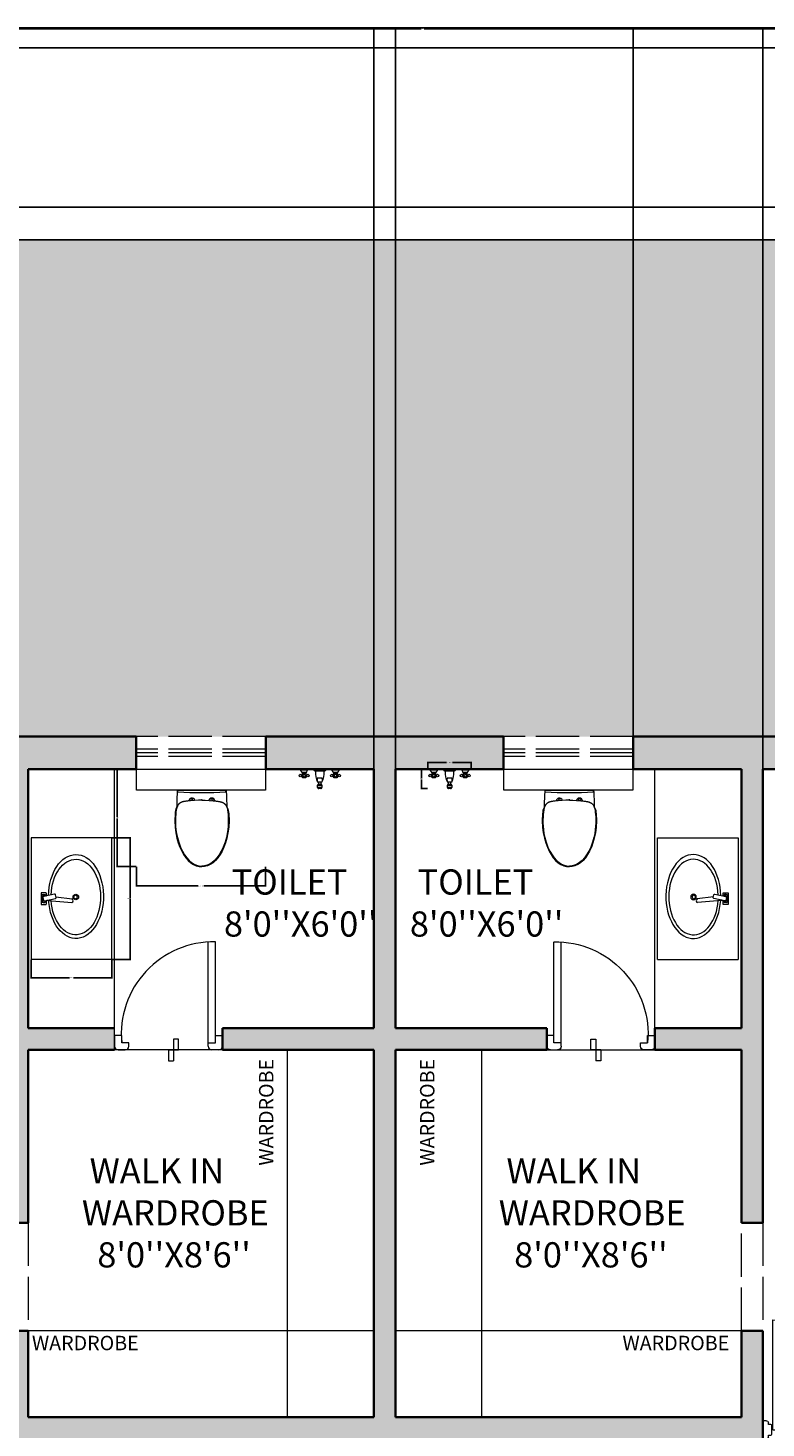
# Model space of a CAD drawing. Units: inches. Extents: x 84 to 1044, y -280 to 906.
# Tile 65 of 105: x 440 to 645, y 517 to 906. Entities that reach past the tile are written whole.
import ezdxf

# ---------------------------------------------------------------- set-up
doc = ezdxf.new("R2010")
doc.units = ezdxf.units.IN
doc.linetypes.add('ACAD_ISO02W100', pattern=[15, 12, -3])
for name, color, linetype, lineweight in [('00 FURNITURE', 15, 'Continuous', 15), ('A-ANNO-DIMS', 2, 'Continuous', 18), ('A-ANNO-TEXT', 7, 'Continuous', 13), ('A-ANNO-TTLB', 7, 'Continuous', 25), ('A-AREA-IDEN', 7, 'Continuous', 13), ('A-DOOR', 4, 'Continuous', 18), ('A-FLOR-CASE', 8, 'Continuous', 18), ('A-FLOR-FIXT', 9, 'Continuous', 15), ('A-GLAZ-HIGH', 160, 'ACAD_ISO02W100', 13), ('A-WALL-OVHD', 8, 'ACAD_ISO02W100', 13), ('A_FUR 1', 5, 'Continuous', 5), ('C-PROP', 7, 'Continuous', 25), ('WALL', 250, 'Continuous', 35)]:
    doc.layers.add(name, color=color, linetype=linetype, lineweight=lineweight)
doc.layers.add('A-WALL-PATT', color=251, linetype='Continuous', lineweight=9, true_color=0x636466)
doc.layers.add('L-PLNT-PATT', color=9, linetype='Continuous', lineweight=9, true_color=0xafd9aa)
doc.styles.add('1-100DIM', font='txt', dxfattribs={"height": 0.3})
doc.styles.get("Standard").update_dxf_attribs({"font": 'arial.ttf'})
doc.dimstyles.get("Standard").update_dxf_attribs({"dimtxt": 0.18, "dimasz": 0.18, "dimexe": 0.18, "dimexo": 0.0625, "dimgap": 0.09, "dimtad": 0, "dimtih": 1, "dimtoh": 1, "dimdec": 4, "dimzin": 0, "dimdsep": 46, "dimtxsty": 'Standard', "dimcen": 0.09, "dimadec": 0, "dimazin": 0, "dimtfac": 1, "dimtdec": 4, "dimtofl": 0, "dimtmove": 0, "dimatfit": 3, "dimfxl": 1, "dimtolj": 1, "dimtzin": 0, "dimarcsym": 0})

# ---------------------------------------------------------------- blocks, each defined once
blk = doc.blocks.new('DDD')
at = {"layer": '00 FURNITURE'}
for p, q in [((-12579.77, -15859.53), (-12579.77, -15829.05)), ((-12578.77, -15859.53), (-12578.77, -15829.03)), ((-12612.02, -15857.03), (-12612.02, -15862.03)), ((-12611.02, -15857.03), (-12612.02, -15857.03)), ((-12610.52, -15858.03), (-12610.52, -15857.53)), ((-12577.52, -15858.03), (-12577.52, -15857.53)), ((-12577.02, -15857.03), (-12576.02, -15857.03)), ((-12576.02, -15857.03), (-12576.02, -15862.03)), ((-12612.02, -15862.03), (-12611.02, -15862.03)), ((-12610.52, -15861.53), (-12610.52, -15861.03)), ((-12578.77, -15859.53), (-12579.77, -15859.53)), ((-12577.52, -15861.53), (-12577.52, -15861.03)), ((-12576.02, -15862.03), (-12577.02, -15862.03))]:
    blk.add_line(p, q, dxfattribs=at)
for points in [[(-12610.52, -15861.03), (-12610.02, -15861.03, 0.414214), (-12609.52, -15860.53), (-12609.52, -15858.53, 0.414214), (-12610.02, -15858.03), (-12610.52, -15858.03)], [(-12577.52, -15861.03), (-12578.02, -15861.03, -0.414214), (-12578.52, -15860.53), (-12578.52, -15858.53, -0.414214), (-12578.02, -15858.03), (-12577.52, -15858.03)]]:
    blk.add_lwpolyline(points, format="xyb", dxfattribs=at)
for centre, radius, start, end in [((-12578.77, -15859.53), 30.5, 90, 180), ((-12611.02, -15857.53), 0.5, 0, 90), ((-12577.02, -15857.53), 0.5, 90, 180), ((-12611.02, -15861.53), 0.5, 270, 0), ((-12577.02, -15861.53), 0.5, 180, 270)]:
    blk.add_arc(centre, radius, start, end, dxfattribs=at)
blk = doc.blocks.new('ESTSET')
at = {"layer": 'A_FUR 1'}
for p, q in [((-10.44, 4.1), (-10.44, 32.1)), ((-8.44, 4.1), (-8.44, 32.1)), ((-36.44, 6.1), (-36.44, 3.1)), ((-34.44, 6.1), (-36.44, 6.1)), ((-34.44, 4.1), (-34.44, 6.1)), ((-34.44, 4.1), (-34.44, 6.1)), ((-32.44, 4.1), (-34.44, 4.1)), ((-32.44, 4.1), (-34.44, 4.1)), ((-32.44, 3.1), (-32.44, 4.1)), ((-10.44, 3.1), (-10.44, 4.1)), ((-10.44, 4.1), (-8.44, 4.1)), ((-10.44, 4.1), (-8.44, 4.1)), ((-8.44, 4.1), (-8.44, 6.1)), ((-8.44, 6.1), (-6.44, 6.1)), ((-8.44, 4.1), (-8.44, 6.1)), ((-6.44, 6.1), (-6.44, 3.1)), ((-6.44, 2.1), (-36.44, 2.1)), ((-35.44, 2.1), (-33.44, 2.1)), ((-7.44, 2.1), (-9.44, 2.1))]:
    blk.add_line(p, q, dxfattribs=at)
for points in [[(-21.44, 2.1), (-18.67, 2.1), (-18.67, 5.1), (-20.06, 5.1)], [(-20.06, 5.1), (-20.06, -0.91)], [(-21.44, 2.1), (-21.44, -0.91), (-20.06, -0.91)]]:
    blk.add_lwpolyline(points, dxfattribs=at)
for centre, radius, start, end in [((-8.91, 6.46), 25.64, 88.9606, 185.2816), ((-35.44, 3.1), 1, 180, 270), ((-33.44, 3.1), 1, 270, 0), ((-9.44, 3.1), 1, 180, 270), ((-7.44, 3.1), 1, 270, 0)]:
    blk.add_arc(centre, radius, start, end, dxfattribs=at)
blk = doc.blocks.new('32')
at = {"layer": '00 FURNITURE'}
for p, q in [((-6.82, 0), (6.82, 0)), ((-6.68, -0.51), (-6.68, 0)), ((6.24, 0), (6.68, 0)), ((6.68, -0.51), (6.68, 0)), ((-6.41, -3.88), (-6.45, -3.92)), ((-6.38, -3.85), (-6.41, -3.88)), ((-6.34, -3.81), (-6.38, -3.85)), ((-6.31, -3.78), (-6.34, -3.81)), ((-6.27, -3.75), (-6.31, -3.78)), ((-6.24, -3.72), (-6.27, -3.75)), ((-6.2, -3.69), (-6.24, -3.72)), ((-6.16, -3.66), (-6.2, -3.69)), ((-6.13, -3.63), (-6.16, -3.66)), ((-6.09, -3.61), (-6.13, -3.63)), ((-6.05, -3.58), (-6.09, -3.61)), ((-6.01, -3.56), (-6.05, -3.58)), ((-5.98, -3.53), (-6.01, -3.56)), ((-5.94, -3.51), (-5.98, -3.53)), ((-5.91, -3.49), (-5.94, -3.51)), ((-5.87, -3.47), (-5.91, -3.49)), ((-5.83, -3.46), (-5.87, -3.47)), ((-5.8, -3.44), (-5.83, -3.46)), ((-5.76, -3.42), (-5.8, -3.44)), ((-5.73, -3.41), (-5.76, -3.42)), ((-5.7, -3.39), (-5.73, -3.41)), ((-5.66, -3.38), (-5.7, -3.39)), ((-5.63, -3.36), (-5.66, -3.38)), ((-5.6, -3.35), (-5.63, -3.36)), ((-5.57, -3.34), (-5.6, -3.35)), ((-5.53, -3.33), (-5.57, -3.34)), ((-5.5, -3.32), (-5.53, -3.33)), ((-5.47, -3.31), (-5.5, -3.32)), ((-5.44, -3.3), (-5.47, -3.31)), ((-5.41, -3.29), (-5.44, -3.3)), ((-5.39, -3.28), (-5.41, -3.29)), ((-5.36, -3.27), (-5.39, -3.28)), ((-5.33, -3.26), (-5.36, -3.27)), ((-5.3, -3.26), (-5.33, -3.26)), ((-5.27, -3.25), (-5.3, -3.26)), ((-5.25, -3.24), (-5.27, -3.25)), ((-5.22, -3.24), (-5.25, -3.24)), ((-5.19, -3.23), (-5.22, -3.24)), ((-5.17, -3.22), (-5.19, -3.23)), ((-5.15, -3.22), (-5.17, -3.22)), ((-5.12, -3.21), (-5.15, -3.22)), ((-5.1, -3.21), (-5.12, -3.21)), ((-5.08, -3.2), (-5.1, -3.21)), ((-5.05, -3.2), (-5.08, -3.2)), ((-5.03, -3.2), (-5.05, -3.2)), ((-5.01, -3.19), (-5.03, -3.2)), ((-4.97, -3.19), (-5.01, -3.19)), ((-4.93, -3.18), (-4.97, -3.19)), ((-4.89, -3.17), (-4.93, -3.18)), ((-4.86, -3.17), (-4.89, -3.17)), ((-4.82, -3.16), (-4.86, -3.17)), ((-4.78, -3.15), (-4.82, -3.16)), ((-4.72, -3.15), (-4.78, -3.15)), ((-4.63, -3.13), (-4.72, -3.15)), ((-4.46, -3.11), (-4.64, -3.14)), ((-4.34, -3.09), (-4.46, -3.11)), ((-4.15, -3.07), (-4.34, -3.09)), ((-3.99, -3.05), (-4.15, -3.07)), ((-3.77, -3.02), (-3.99, -3.05)), ((-3.5, -2.99), (-3.77, -3.02)), ((-3.34, -2.97), (-3.5, -2.99)), ((-3.3, -2.97), (-3.32, -2.97)), ((-3.26, -2.96), (-3.3, -2.97)), ((-3.21, -2.96), (-3.26, -2.96)), ((-3.15, -2.95), (-3.2, -2.96)), ((-2.01, -2.84), (-3.15, -2.95)), ((-0.94, -2.78), (-2.01, -2.84)), ((0, -2.76), (-0.94, -2.78)), ((0.12, -2.71), (-0.12, -2.71)), ((0, -2.76), (0.94, -2.78)), ((0.94, -2.78), (2.01, -2.84)), ((2.01, -2.84), (3.15, -2.95)), ((3.15, -2.95), (3.2, -2.96)), ((3.21, -2.96), (3.26, -2.96)), ((3.26, -2.96), (3.3, -2.97)), ((3.3, -2.97), (3.32, -2.97)), ((3.34, -2.97), (3.5, -2.99)), ((3.5, -2.99), (3.77, -3.02)), ((3.77, -3.02), (3.99, -3.05)), ((3.99, -3.05), (4.15, -3.07)), ((4.15, -3.07), (4.34, -3.09)), ((4.34, -3.09), (4.46, -3.11)), ((4.46, -3.11), (4.64, -3.14)), ((4.63, -3.13), (4.72, -3.15)), ((4.72, -3.15), (4.78, -3.15)), ((4.78, -3.15), (4.82, -3.16)), ((4.82, -3.16), (4.86, -3.17)), ((4.86, -3.17), (4.89, -3.17)), ((4.89, -3.17), (4.93, -3.18)), ((4.93, -3.18), (4.97, -3.19)), ((4.97, -3.19), (5.01, -3.19)), ((5.01, -3.19), (5.03, -3.2)), ((5.03, -3.2), (5.05, -3.2)), ((5.05, -3.2), (5.08, -3.2)), ((5.08, -3.2), (5.1, -3.21)), ((5.1, -3.21), (5.12, -3.21)), ((5.12, -3.21), (5.15, -3.22)), ((5.15, -3.22), (5.17, -3.22)), ((5.17, -3.22), (5.19, -3.23)), ((5.19, -3.23), (5.22, -3.24)), ((5.22, -3.24), (5.25, -3.24)), ((5.25, -3.24), (5.27, -3.25)), ((5.27, -3.25), (5.3, -3.26)), ((5.3, -3.26), (5.33, -3.26)), ((5.33, -3.26), (5.36, -3.27)), ((5.36, -3.27), (5.39, -3.28)), ((5.39, -3.28), (5.41, -3.29)), ((5.41, -3.29), (5.44, -3.3)), ((5.44, -3.3), (5.47, -3.31)), ((5.47, -3.31), (5.5, -3.32)), ((5.5, -3.32), (5.53, -3.33)), ((5.53, -3.33), (5.57, -3.34)), ((5.57, -3.34), (5.6, -3.35)), ((5.6, -3.35), (5.63, -3.36)), ((5.63, -3.36), (5.66, -3.38)), ((5.66, -3.38), (5.7, -3.39)), ((5.7, -3.39), (5.73, -3.41)), ((5.73, -3.41), (5.76, -3.42)), ((5.76, -3.42), (5.8, -3.44)), ((5.8, -3.44), (5.83, -3.46)), ((5.83, -3.46), (5.87, -3.47)), ((5.87, -3.47), (5.91, -3.49)), ((5.91, -3.49), (5.94, -3.51)), ((5.94, -3.51), (5.98, -3.53)), ((5.98, -3.53), (6.01, -3.56)), ((6.01, -3.56), (6.05, -3.58)), ((6.05, -3.58), (6.09, -3.61)), ((6.09, -3.61), (6.13, -3.63)), ((6.13, -3.63), (6.16, -3.66)), ((6.16, -3.66), (6.2, -3.69)), ((6.2, -3.69), (6.24, -3.72)), ((6.24, -3.72), (6.27, -3.75)), ((6.27, -3.75), (6.31, -3.78)), ((6.31, -3.78), (6.34, -3.81)), ((6.34, -3.81), (6.38, -3.85)), ((6.38, -3.85), (6.41, -3.88)), ((6.41, -3.88), (6.45, -3.92)), ((-7.44, -6.63), (-7.53, -8.53)), ((-7.39, -6.15), (-7.44, -6.62)), ((-7.32, -5.67), (-7.39, -6.15)), ((-7.31, -7.51), (-7.34, -8.28)), ((-7.21, -5.24), (-7.32, -5.67)), ((-7.27, -6.79), (-7.31, -7.51)), ((-7.21, -6.12), (-7.27, -6.79)), ((-7.01, -4.86), (-7.21, -5.24)), ((-7.13, -5.49), (-7.21, -6.12)), ((-6.99, -4.9), (-7.13, -5.49)), ((-6.93, -4.76), (-7.01, -4.86)), ((-6.79, -4.42), (-6.99, -4.9)), ((-6.77, -4.39), (-6.79, -4.42)), ((-6.74, -4.33), (-6.77, -4.39)), ((-6.71, -4.28), (-6.74, -4.33)), ((-6.67, -4.22), (-6.71, -4.28)), ((-6.64, -4.17), (-6.67, -4.22)), ((-6.61, -4.13), (-6.64, -4.17)), ((-6.58, -4.08), (-6.61, -4.13)), ((-6.55, -4.04), (-6.58, -4.08)), ((-6.51, -4), (-6.55, -4.04)), ((-6.48, -3.96), (-6.51, -4)), ((-6.45, -3.92), (-6.48, -3.96)), ((6.45, -3.92), (6.48, -3.96)), ((6.48, -3.96), (6.51, -4)), ((6.51, -4), (6.55, -4.04)), ((6.55, -4.04), (6.58, -4.08)), ((6.58, -4.08), (6.61, -4.13)), ((6.61, -4.13), (6.64, -4.17)), ((6.64, -4.17), (6.67, -4.22)), ((6.67, -4.22), (6.71, -4.28)), ((6.71, -4.28), (6.74, -4.33)), ((6.74, -4.33), (6.77, -4.39)), ((6.77, -4.39), (6.79, -4.42)), ((6.79, -4.42), (6.99, -4.9)), ((6.93, -4.76), (7.01, -4.86)), ((6.99, -4.9), (7.13, -5.49)), ((7.01, -4.86), (7.21, -5.24)), ((7.13, -5.49), (7.21, -6.12)), ((7.21, -5.24), (7.32, -5.67)), ((7.21, -6.12), (7.27, -6.79)), ((7.27, -6.79), (7.31, -7.51)), ((7.31, -7.51), (7.34, -8.28)), ((7.32, -5.67), (7.39, -6.15)), ((7.39, -6.15), (7.44, -6.62)), ((7.44, -6.63), (7.53, -8.53)), ((-7.53, -8.53), (-7.45, -10.3)), ((-7.45, -10.3), (-7.24, -11.89)), ((-7.34, -8.28), (-7.34, -9.11)), ((-7.34, -9.11), (-7.3, -10)), ((-7.3, -10), (-7.21, -10.97)), ((-7.21, -10.97), (-7.06, -12.03)), ((7.21, -10.97), (7.06, -12.03)), ((7.3, -10), (7.21, -10.97)), ((7.45, -10.3), (7.24, -11.89)), ((7.34, -9.11), (7.3, -10)), ((7.34, -8.28), (7.34, -9.11)), ((7.53, -8.53), (7.45, -10.3)), ((-7.24, -11.89), (-6.93, -13.34)), ((-7.06, -12.03), (-6.81, -13.19)), ((-6.93, -13.34), (-6.55, -14.65)), ((-6.81, -13.19), (-6.44, -14.48)), ((-6.55, -14.65), (-6.11, -15.85)), ((-6.44, -14.48), (-5.95, -15.8)), ((6.44, -14.48), (5.95, -15.8)), ((6.55, -14.65), (6.11, -15.85)), ((6.81, -13.19), (6.44, -14.48)), ((6.93, -13.34), (6.55, -14.65)), ((7.06, -12.03), (6.81, -13.19)), ((7.24, -11.89), (6.93, -13.34)), ((-6.11, -15.85), (-5.61, -16.94)), ((-5.95, -15.8), (-5.38, -16.99)), ((-5.61, -16.94), (-5.06, -17.92)), ((-5.38, -16.99), (-4.79, -17.98)), ((-5.06, -17.92), (-4.45, -18.78)), ((-4.79, -17.98), (-4.17, -18.83)), ((-4.45, -18.78), (-3.8, -19.54)), ((-4.17, -18.83), (-3.53, -19.54)), ((4.17, -18.83), (3.53, -19.54)), ((4.45, -18.78), (3.8, -19.54)), ((4.79, -17.98), (4.17, -18.83)), ((5.06, -17.92), (4.45, -18.78)), ((5.38, -16.99), (4.79, -17.98)), ((5.61, -16.94), (5.06, -17.92)), ((5.95, -15.8), (5.38, -16.99)), ((6.11, -15.85), (5.61, -16.94)), ((-3.8, -19.54), (-3.09, -20.17)), ((-3.53, -19.54), (-2.86, -20.12)), ((-3.09, -20.17), (-2.34, -20.67)), ((-2.86, -20.12), (-2.18, -20.55)), ((-2.34, -20.67), (-1.55, -21.01)), ((-2.18, -20.55), (-1.47, -20.85)), ((-1.55, -21.01), (-0.75, -21.2)), ((-1.47, -20.85), (-0.74, -21.03)), ((-0.75, -21.2), (0, -21.25)), ((-0.74, -21.03), (0, -21.08)), ((0.74, -21.03), (0, -21.08)), ((0.75, -21.2), (0, -21.25)), ((1.47, -20.85), (0.74, -21.03)), ((1.55, -21.01), (0.75, -21.2)), ((2.18, -20.55), (1.47, -20.85)), ((2.34, -20.67), (1.55, -21.01)), ((2.86, -20.12), (2.18, -20.55)), ((3.09, -20.17), (2.34, -20.67)), ((3.53, -19.54), (2.86, -20.12)), ((3.8, -19.54), (3.09, -20.17))]:
    blk.add_line(p, q, dxfattribs=at)
for points in [[(-6.82, 0), (-6.91, -1.63), (-6.97, -3.26), (-7.01, -4.89)], [(7.01, -4.89), (6.97, -3.26), (6.91, -1.63), (6.82, 0)], [(-6.68, -0.51), (-2.23, -0.73), (2.23, -0.73), (6.68, -0.51)], [(-2.97, -2.23), (-3.33, -2.32), (-3.59, -2.63), (-3.61, -3)], [(-1.94, -2.84), (-2.06, -2.38), (-2.52, -2.11), (-2.97, -2.23)], [(-2.58, -2.49), (-2.63, -2.45), (-2.7, -2.43), (-2.76, -2.43)], [(-2.54, -2.89), (-2.44, -2.77), (-2.46, -2.59), (-2.58, -2.49)], [(2.76, -2.2), (2.38, -2.2), (2.04, -2.46), (1.94, -2.84)], [(3.61, -3), (3.58, -2.55), (3.21, -2.2), (2.76, -2.2)], [(2.98, -2.53), (2.93, -2.46), (2.85, -2.43), (2.76, -2.43)], [(2.95, -2.93), (3.07, -2.83), (3.08, -2.65), (2.98, -2.53)]]:
    blk.add_open_spline(points, degree=3, dxfattribs=at)
for points in [[(-2.76, -2.43), (-2.92, -2.43), (-3.05, -2.56), (-3.05, -2.71), (-3.05, -2.8), (-3.01, -2.88), (-2.95, -2.93)], [(2.76, -2.43), (2.6, -2.43), (2.48, -2.56), (2.48, -2.71), (2.48, -2.78), (2.5, -2.84), (2.54, -2.89)]]:
    blk.add_open_spline(points, degree=3, knots=[0, 0, 0, 0, 1, 1, 1, 2, 2, 2, 2], dxfattribs=at)
blk = doc.blocks.new('WWCC')
at = {"layer": '00 FURNITURE', "ltscale": 20}
blk.add_lwpolyline([(140241.58, -48678.24), (140247.43, -48678.24), (140247.43, -48714.06), (140241.58, -48714.06)], close=True, dxfattribs=at)
at = {"layer": '00 FURNITURE', "rotation": 90.00000000000003}
blk.add_blockref('32', (140247.43, -48695.89), dxfattribs=at)
blk = doc.blocks.new('Faucet - Bathroom front')
for p, q in [((-0.5, 4.25), (0.5, 4.25)), ((0.5, 3.75), (-0.5, 3.75)), ((-0.25, 3), (-0.25, 3.5)), ((0.25, 3.5), (0.25, 3)), ((-5, 0), (-2.25, 0)), ((-4.5087, 0.25), (-2.7408, 0.25)), ((-4, 1.625), (-4.25, 1.625)), ((-4, 1.375), (-4.25, 1.375)), ((-3.1442, 0.75), (-4.0979, 0.75)), ((-3.25, 1.625), (-3, 1.625)), ((-3.25, 1.375), (-3, 1.375)), ((-1.5, 0), (1.5, 0)), ((-1, 0.5), (1, 0.5)), ((-0.5, 3), (0.5, 3)), ((0.5, 2), (-0.5, 2)), ((2.25, 0), (5, 0)), ((2.7413, 0.25), (4.5092, 0.25)), ((3.25, 1.625), (3, 1.625)), ((3.25, 1.375), (3, 1.375)), ((4.1058, 0.75), (3.1521, 0.75)), ((4, 1.625), (4.25, 1.625)), ((4, 1.375), (4.25, 1.375))]:
    blk.add_line(p, q)
for points in [[(-0.5, 3.75), (-0.5, 4.25)], [(-0.25, 4.5), (0.25, 4.5)], [(0.25, 3.5), (-0.25, 3.5)], [(0.5, 4.25), (0.5, 3.75)]]:
    blk.add_lwpolyline(points)
for points in [[(-4, 1), (-4, 2), (-3.25, 2), (-3.25, 1)], [(3.25, 1), (3.25, 2), (4, 2), (4, 1)]]:
    blk.add_lwpolyline(points, close=True)
for centre in [(-4.5, 1.5), (-3.625, 1.5), (-2.75, 1.5), (2.75, 1.5), (3.625, 1.5), (4.5, 1.5)]:
    blk.add_circle(centre, 0.2795)
for centre, radius, start, end in [((-0.2575, 4.2575), 0.2426, 88.22243, 181.7776), ((-0.2575, 3.7425), 0.2426, 178.2224, 271.7776), ((0.2575, 4.2575), 0.2426, 358.2224, 91.77757), ((0.2575, 3.7425), 0.2426, 268.2224, 1.777565), ((-5.375, 1.375), 1.4252, 285.2551, 344.7449), ((-1.875, 1.375), 1.4252, 195.2551, 254.7449), ((-0.7962, -0.2038), 0.7327, 106.1502, 163.8498), ((3, 1), 4.0311, 150.2551, 187.125), ((0.6413, 2.5), 1.246, 156.3417, 203.6583), ((-3, 1), 4.0311, 352.875, 29.74488), ((-0.6413, 2.5), 1.246, 336.3417, 23.65835), ((0.7962, -0.2038), 0.7327, 16.1502, 73.84979), ((1.875, 1.375), 1.4252, 285.2551, 344.7449), ((5.375, 1.375), 1.4252, 195.2551, 254.7449)]:
    blk.add_arc(centre, radius, start, end)
blk = doc.blocks.new('VANITY-BOWL-COUNTER')
for p, q in [((0, 33.78), (0, 0)), ((22.37, 33.78), (0, 33.78)), ((22.37, 0), (22.37, 33.78)), ((22.37, 0), (0, 0))]:
    blk.add_line(p, q)
for centre, radius in [((12.39, 17.35), 0.775), ((12.39, 17.35), 0.775), ((12.3, 17.36), 0.488)]:
    blk.add_circle(centre, radius)
at = {"extrusion": (0, 0, -1)}
for centre, major_axis, start_param, end_param in [((12.43, 17.49), (0, 11.65), -1.54793, 4.618862), ((12.39, 17.35), (0, 10.49), -1.516557, 4.61628)]:
    blk.add_ellipse(centre, major_axis=major_axis, ratio=0.654321, start_param=start_param, end_param=end_param, dxfattribs=at)
blk = doc.blocks.new('WIN-HIGH-36IN')
for p, q in [((3.5, 36), (3.5, 0)), ((4.5, 36), (4.5, 0)), ((5.5, 36), (5.5, 0))]:
    blk.add_line(p, q)
blk.add_lwpolyline([(0, 0), (9, 0), (9, 36), (0, 36)], close=True)
blk = doc.blocks.new('*D44')
at = {"layer": 'A-ANNO-DIMS', "color": 0, "lineweight": -2, "transparency": 16777216}
for p, q in [((470.16, 672.95), (470.16, 667.46)), ((505.98, 672.95), (505.98, 667.46)), ((470.34, 667.64), (487.3, 667.64)), ((505.8, 667.64), (488.85, 667.64))]:
    blk.add_line(p, q, dxfattribs=at)
at = {"layer": 'A-ANNO-DIMS', "color": 0, "transparency": 16777216}
for points in [[(470.34, 667.67), (470.34, 667.61), (470.16, 667.64)], [(505.8, 667.67), (505.8, 667.61), (505.98, 667.64)]]:
    blk.add_solid(points, dxfattribs=at)
at = {"layer": 'Defpoints', "color": 0, "transparency": 16777216}
for p in [(470.16, 673.02), (505.98, 673.02), (505.98, 667.64)]:
    blk.add_point(p, dxfattribs=at)
at = {"layer": 'A-ANNO-DIMS', "color": 0, "transparency": 16777216, "insert": (488.07, 667.64), "char_height": 0.18, "attachment_point": 5}
blk.add_mtext('\\A1;WC 36 TYP.', dxfattribs=at)
blk = doc.blocks.new('*D45')
at = {"layer": 'A-ANNO-DIMS', "color": 0, "lineweight": -2, "transparency": 16777216}
for p, q in [((470.1, 700.12), (464.61, 700.12)), ((464.79, 699.94), (464.79, 686.75)), ((464.79, 673.2), (464.79, 686.39)), ((470.1, 673.02), (464.61, 673.02))]:
    blk.add_line(p, q, dxfattribs=at)
at = {"layer": 'A-ANNO-DIMS', "color": 0, "transparency": 16777216}
for points in [[(464.76, 699.94), (464.82, 699.94), (464.79, 700.12)], [(464.76, 673.2), (464.82, 673.2), (464.79, 673.02)]]:
    blk.add_solid(points, dxfattribs=at)
at = {"layer": 'Defpoints', "color": 0, "transparency": 16777216}
for p in [(470.16, 700.12), (464.79, 673.02), (470.16, 673.02)]:
    blk.add_point(p, dxfattribs=at)
at = {"layer": 'A-ANNO-DIMS', "color": 0, "transparency": 16777216, "insert": (464.79, 686.57), "char_height": 0.18, "attachment_point": 5}
blk.add_mtext('\\A1;27 TYP.', dxfattribs=at)
blk = doc.blocks.new('*D46')
at = {"layer": 'A-ANNO-DIMS', "color": 0, "lineweight": -2, "transparency": 16777216}
for p, q in [((463.39, 681.01), (468.58, 681.01)), ((468.4, 680.83), (468.4, 664.3)), ((468.4, 647.41), (468.4, 663.94)), ((463.39, 647.23), (468.58, 647.23))]:
    blk.add_line(p, q, dxfattribs=at)
at = {"layer": 'A-ANNO-DIMS', "color": 0, "transparency": 16777216}
for points in [[(468.37, 680.83), (468.43, 680.83), (468.4, 681.01)], [(468.37, 647.41), (468.43, 647.41), (468.4, 647.23)]]:
    blk.add_solid(points, dxfattribs=at)
at = {"layer": 'Defpoints', "color": 0, "transparency": 16777216}
for p in [(463.33, 681.01), (468.4, 681.01), (463.33, 647.23)]:
    blk.add_point(p, dxfattribs=at)
at = {"layer": 'A-ANNO-DIMS', "color": 0, "transparency": 16777216, "insert": (468.4, 664.12), "char_height": 0.18, "attachment_point": 5}
blk.add_mtext('\\A1;VANITY 34 TYP.', dxfattribs=at)
blk = doc.blocks.new('*D47')
at = {"layer": 'A-ANNO-DIMS', "color": 0, "lineweight": -2, "transparency": 16777216}
for p, q in [((440.96, 647.16), (440.96, 641.98)), ((463.33, 647.16), (463.33, 641.98)), ((441.14, 642.16), (451.62, 642.16)), ((463.15, 642.16), (452.67, 642.16))]:
    blk.add_line(p, q, dxfattribs=at)
at = {"layer": 'A-ANNO-DIMS', "color": 0, "transparency": 16777216}
for points in [[(441.14, 642.19), (441.14, 642.13), (440.96, 642.16)], [(463.15, 642.19), (463.15, 642.13), (463.33, 642.16)]]:
    blk.add_solid(points, dxfattribs=at)
at = {"layer": 'Defpoints', "color": 0, "transparency": 16777216}
for p in [(440.96, 647.23), (463.33, 647.23), (463.33, 642.16)]:
    blk.add_point(p, dxfattribs=at)
at = {"layer": 'A-ANNO-DIMS', "color": 0, "transparency": 16777216, "insert": (452.15, 642.16), "char_height": 0.18, "attachment_point": 5}
blk.add_mtext('\\A1;22 TYP.', dxfattribs=at)
blk = doc.blocks.new('*D48')
at = {"layer": 'A-ANNO-DIMS', "color": 0, "lineweight": -2, "transparency": 16777216}
for p, q in [((551.06, 700.18), (551.06, 702.1)), ((551.24, 701.92), (556.26, 701.92)), ((562.91, 701.92), (557.88, 701.92)), ((563.09, 700.18), (563.09, 702.1))]:
    blk.add_line(p, q, dxfattribs=at)
at = {"layer": 'A-ANNO-DIMS', "color": 0, "transparency": 16777216}
for points in [[(551.24, 701.95), (551.24, 701.89), (551.06, 701.92)], [(562.91, 701.95), (562.91, 701.89), (563.09, 701.92)]]:
    blk.add_solid(points, dxfattribs=at)
at = {"layer": 'Defpoints', "color": 0, "transparency": 16777216}
for p in [(551.06, 701.92), (551.06, 700.12), (563.09, 700.12)]:
    blk.add_point(p, dxfattribs=at)
at = {"layer": 'A-ANNO-DIMS', "color": 0, "transparency": 16777216, "insert": (557.07, 701.92), "char_height": 0.18, "attachment_point": 5}
blk.add_mtext('\\A1;TAP 12 TYP.', dxfattribs=at)
blk = doc.blocks.new('*D49')
at = {"layer": 'A-ANNO-DIMS', "color": 0, "lineweight": -2, "transparency": 16777216}
for p, q in [((551, 700.12), (549.07, 700.12)), ((549.25, 699.94), (549.25, 697.59)), ((549.25, 694.88), (549.25, 697.23)), ((551, 694.7), (549.07, 694.7))]:
    blk.add_line(p, q, dxfattribs=at)
at = {"layer": 'A-ANNO-DIMS', "color": 0, "transparency": 16777216}
for points in [[(549.22, 699.94), (549.28, 699.94), (549.25, 700.12)], [(549.22, 694.88), (549.28, 694.88), (549.25, 694.7)]]:
    blk.add_solid(points, dxfattribs=at)
at = {"layer": 'Defpoints', "color": 0, "transparency": 16777216}
for p in [(551.06, 700.12), (549.25, 694.7), (551.06, 694.7)]:
    blk.add_point(p, dxfattribs=at)
at = {"layer": 'A-ANNO-DIMS', "color": 0, "transparency": 16777216, "insert": (549.25, 697.41), "char_height": 0.18, "attachment_point": 5}
blk.add_mtext('\\A1;5 TYP.', dxfattribs=at)
blk = doc.blocks.new('*D62')
at = {"layer": 'A-ANNO-DIMS', "color": 0, "lineweight": -2, "transparency": 16777216}
for p, q in [((203.18, 709.18), (203.18, 905.9)), ((896.07, 400.18), (896.07, 905.9)), ((203.36, 905.72), (549.23, 905.72)), ((895.89, 905.72), (550.02, 905.72))]:
    blk.add_line(p, q, dxfattribs=at)
at = {"layer": 'A-ANNO-DIMS', "color": 0, "transparency": 16777216}
for points in [[(203.36, 905.75), (203.36, 905.69), (203.18, 905.72)], [(895.89, 905.75), (895.89, 905.69), (896.07, 905.72)]]:
    blk.add_solid(points, dxfattribs=at)
at = {"layer": 'Defpoints', "color": 0, "transparency": 16777216}
for p in [(896.07, 905.72), (203.18, 709.12), (896.07, 400.12)]:
    blk.add_point(p, dxfattribs=at)
at = {"layer": 'A-ANNO-DIMS', "color": 0, "transparency": 16777216, "insert": (549.63, 905.72), "char_height": 0.18, "attachment_point": 5}
blk.add_mtext('\\A1;692.9', dxfattribs=at)
blk = doc.blocks.new('*D73')
at = {"layer": 'A-ANNO-DIMS', "color": 0, "lineweight": -2, "transparency": 16777216}
for p, q in [((536.07, 700.18), (536.07, 905.9)), ((542.07, 700.18), (542.07, 905.9)), ((536.25, 905.72), (538.92, 905.72)), ((541.89, 905.72), (539.22, 905.72))]:
    blk.add_line(p, q, dxfattribs=at)
at = {"layer": 'A-ANNO-DIMS', "color": 0, "transparency": 16777216}
for points in [[(536.25, 905.75), (536.25, 905.69), (536.07, 905.72)], [(541.89, 905.75), (541.89, 905.69), (542.07, 905.72)]]:
    blk.add_solid(points, dxfattribs=at)
at = {"layer": 'Defpoints', "color": 0, "transparency": 16777216}
for p in [(542.07, 905.72), (536.07, 700.12), (542.07, 700.12)]:
    blk.add_point(p, dxfattribs=at)
at = {"layer": 'A-ANNO-DIMS', "color": 0, "transparency": 16777216, "insert": (539.07, 905.72), "char_height": 0.18, "attachment_point": 5}
blk.add_mtext('\\A1;6', dxfattribs=at)
blk = doc.blocks.new('*D75')
at = {"layer": 'A-ANNO-DIMS', "color": 0, "lineweight": -2, "transparency": 16777216}
for p, q in [((608.07, 709.18), (608.07, 905.9)), ((644.07, 700.18), (644.07, 905.9)), ((608.25, 905.72), (625.86, 905.72)), ((643.89, 905.72), (626.29, 905.72))]:
    blk.add_line(p, q, dxfattribs=at)
at = {"layer": 'A-ANNO-DIMS', "color": 0, "transparency": 16777216}
for points in [[(608.25, 905.75), (608.25, 905.69), (608.07, 905.72)], [(643.89, 905.75), (643.89, 905.69), (644.07, 905.72)]]:
    blk.add_solid(points, dxfattribs=at)
at = {"layer": 'Defpoints', "color": 0, "transparency": 16777216}
for p in [(644.07, 905.72), (608.07, 709.12), (644.07, 700.12)]:
    blk.add_point(p, dxfattribs=at)
at = {"layer": 'A-ANNO-DIMS', "color": 0, "transparency": 16777216, "insert": (626.07, 905.72), "char_height": 0.18, "attachment_point": 5}
blk.add_mtext('\\A1;36', dxfattribs=at)

msp = doc.modelspace()

# ---------------------------------------------------------------- hatches: boundary and pattern name
at = {"layer": 'A-WALL-PATT', "transparency": 33554597}
h = msp.add_hatch(color=256, dxfattribs=at)
h.dxf.hatch_style = 1
h.paths.add_polyline_path([(671.074, 100.12), (647.074, 100.12), (647.074, 160.12), (641.074, 160.12), (620.824, 160.12), (620.824, 151.12), (638.074, 151.12), (638.074, 91.12), (671.074, 91.12)])
h.paths.add_polyline_path([(791.074, 100.12), (743.074, 100.12), (743.074, 91.12), (791.074, 91.12)])
h.paths.add_polyline_path([(896.074, 346.12), (887.074, 346.12), (887.074, 334.12), (870.955, 334.12), (833.074, 334.12), (804.574, 334.12), (804.574, 328.12), (887.074, 328.12), (887.074, 100.12), (863.074, 100.12), (863.074, 91.12), (896.074, 91.12)])
h.paths.add_polyline_path([(507.574, 154.729), (507.574, 160.12), (464.074, 160.12), (464.074, 247.12), (641.074, 247.12), (641.074, 208.12), (647.074, 208.12), (647.074, 328.12), (659.074, 328.12), (659.074, 334.12), (617.074, 334.12), (617.074, 328.12), (641.074, 328.12), (641.074, 256.12), (545.074, 256.12), (545.074, 328.12), (569.074, 328.12), (569.074, 334.12), (518.074, 334.12), (518.074, 325.12), (536.074, 325.12), (536.074, 256.12), (464.074, 256.12), (464.074, 325.12), (482.074, 325.12), (482.074, 334.12), (455.074, 334.12), (455.074, 160.12), (413.127, 160.12), (413.127, 151.12), (455.074, 151.12), (455.074, 91.12), (464.074, 91.12), (464.074, 151.12), (507.574, 151.12)])
h.paths.add_polyline_path([(572.824, 160.12), (555.574, 160.12), (555.574, 151.12), (572.824, 151.12)], flags=17)
h.paths.add_polyline_path([(341.127, 160.12), (299.179, 160.12), (299.179, 211.12), (294.179, 211.12), (290.179, 211.12), (290.179, 151.12), (341.127, 151.12)])
h.paths.add_polyline_path([(299.179, 256.12), (212.179, 256.12), (212.179, 274.12), (203.179, 274.12), (203.179, 247.12), (299.179, 247.12)])
h.paths.add_polyline_path([(212.179, 514.12), (398.074, 514.12), (398.074, 519.12), (398.074, 520.12), (212.179, 520.12), (212.179, 574.12), (203.179, 574.12), (203.179, 310.12), (212.179, 310.12), (212.179, 328.12), (290.179, 328.12), (290.179, 292.12), (299.179, 292.12), (299.179, 328.12), (332.179, 328.12), (332.179, 334.12), (212.179, 334.12)])
h.paths.add_polyline_path([(287.127, 709.12), (203.179, 709.12), (203.179, 646.12), (212.179, 646.12), (212.179, 700.12), (287.127, 700.12)])
h.paths.add_polyline_path([(470.074, 709.12), (359.127, 709.12), (359.127, 700.12), (434.074, 700.12), (434.074, 574.12), (440.074, 574.12), (440.074, 622.12), (464.074, 622.12), (464.074, 628.12), (440.074, 628.12), (440.074, 700.12), (470.074, 700.12)])
h.paths.add_polyline_path([(572.074, 709.12), (506.074, 709.12), (506.074, 700.12), (536.074, 700.12), (536.074, 628.12), (494.074, 628.12), (494.074, 622.12), (536.074, 622.12), (536.074, 520.12), (440.074, 520.12), (440.074, 544.12), (434.074, 544.12), (434.074, 514.12), (644.074, 514.12), (644.074, 519.12), (644.074, 544.12), (638.074, 544.12), (638.074, 520.12), (542.074, 520.12), (542.074, 622.12), (584.074, 622.12), (584.074, 628.12), (542.074, 628.12), (542.074, 700.12), (572.074, 700.12)])
h.paths.add_polyline_path([(698.074, 709.12), (608.074, 709.12), (608.074, 700.12), (638.074, 700.12), (638.074, 628.12), (614.074, 628.12), (614.074, 622.12), (638.074, 622.12), (638.074, 574.12), (644.074, 574.12), (644.074, 700.12), (698.074, 700.12)])
h.paths.add_polyline_path([(833.074, 709.12), (770.074, 709.12), (770.074, 700.12), (824.074, 700.12), (824.074, 646.12), (833.074, 646.12)])
h.paths.add_polyline_path([(833.074, 574.12), (824.074, 574.12), (824.074, 520.12), (791.244, 520.12), (712.904, 520.12), (680.074, 520.12), (680.074, 514.12), (695.074, 514.12), (695.074, 491.62), (704.074, 491.62), (704.074, 511.12), (833.074, 511.12)])
h.paths.add_polyline_path([(704.074, 419.62), (695.074, 419.62), (695.074, 370.12), (704.074, 370.12)])
h.paths.add_polyline_path([(896.074, 400.12), (833.074, 400.12), (833.074, 364.12), (839.074, 364.12), (839.074, 394.12), (887.074, 394.12), (887.074, 382.12), (896.074, 382.12)])
h.paths.add_polyline_path([(732.574, 334.12), (695.074, 334.12), (695.074, 328.12), (732.574, 328.12)])
at = {"layer": 'L-PLNT-PATT', "transparency": 33554597}
h = msp.add_hatch(color=256, dxfattribs=at)
h.dxf.hatch_style = 1
h.paths.add_polyline_path([(434.074, 769.12), (386.074, 769.12), (386.074, 709.12), (434.074, 709.12)])
h.paths.add_polyline_path([(896.074, 847.12), (434.074, 847.12), (434.074, 769.12), (434.074, 709.12), (470.074, 709.12), (506.074, 709.12), (572.074, 709.12), (608.074, 709.12), (698.074, 709.12), (770.074, 709.12), (833.074, 709.12), (896.074, 709.12)])
h.paths.add_polyline_path([(983.074, 847.12), (896.074, 847.12), (896.074, 709.12), (896.074, 547.12), (932.074, 547.12), (983.074, 547.12)])
h.paths.add_polyline_path([(983.074, 547.12), (932.074, 547.12), (932.074, 265.12), (983.074, 265.12)])
h.paths.add_polyline_path([(203.179, 646.12), (203.179, 709.12), (203.179, 745.12), (143.179, 745.12), (143.179, 271.12), (203.179, 271.12), (203.179, 274.12), (203.179, 310.12), (203.179, 574.12)])

# ---------------------------------------------------------------- linework, layer by layer
at = {"layer": 'A-ANNO-TTLB'}
for points in [[(101.1, 905.916), (1027.308, 905.916), (1027.308, -279.764), (101.1, -279.764)], [(106.576, 900.439), (1021.832, 900.439), (1021.832, -274.288), (106.576, -274.288)]]:
    msp.add_lwpolyline(points, close=True, dxfattribs=at)
at = {"layer": 'A-FLOR-CASE'}
for p, q in [((464.074, 622.12), (464.074, 700.12)), ((614.074, 628.12), (614.074, 700.12)), ((512.074, 520.12), (512.074, 622.12)), ((566.074, 520.12), (566.074, 622.12)), ((536.074, 544.12), (440.074, 544.12)), ((638.074, 544.12), (542.074, 544.12))]:
    msp.add_line(p, q, dxfattribs=at)
at = {"layer": 'A-FLOR-FIXT'}
for p, q in [((443.917, 663.46), (443.917, 664.936)), ((444.292, 665.311), (444.731, 665.311)), ((633.856, 665.311), (633.417, 665.311)), ((634.231, 663.46), (634.231, 664.936)), ((444.292, 663.085), (444.707, 663.085)), ((445.596, 663.654), (452.234, 663.08)), ((447.816, 664.638), (452.334, 664.064)), ((630.332, 664.638), (625.814, 664.064)), ((632.552, 663.654), (625.914, 663.08)), ((633.856, 663.085), (633.441, 663.085))]:
    msp.add_line(p, q, dxfattribs=at)
for points in [[(445.16, 664.859), (445.16, 665.589, 0.4142136), (444.973, 665.776), (443.897, 665.776, 0.4142136), (443.71, 665.589), (443.71, 662.651, 0.4142136), (443.897, 662.464), (444.973, 662.464, 0.4142136), (445.16, 662.651), (445.16, 663.483)], [(632.988, 664.859), (632.988, 665.589, -0.4142136), (633.175, 665.776), (634.251, 665.776, -0.4142136), (634.438, 665.589), (634.438, 662.651, -0.4142136), (634.251, 662.464), (633.175, 662.464, -0.4142136), (632.988, 662.651), (632.988, 663.483)]]:
    msp.add_lwpolyline(points, format="xyb", dxfattribs=at)
for points in [[(444.618, 663.526), (447.719, 664.201, 0.4142136), (447.862, 664.424), (447.69, 665.217, 0.4142136), (447.466, 665.361), (444.366, 664.686, 0.4142136), (444.223, 664.463), (444.395, 663.67, 0.4142136)], [(633.53, 663.526), (630.429, 664.201, -0.4142136), (630.286, 664.424), (630.458, 665.217, -0.4142136), (630.681, 665.361), (633.782, 664.686, -0.4142136), (633.925, 664.463), (633.753, 663.67, -0.4142136)]]:
    msp.add_lwpolyline(points, format="xyb", close=True, dxfattribs=at)
for centre, radius, start, end in [((444.292, 664.936), 0.375, 90, 180), ((446.041, 666.147), 1.554, 212.56997, 235.87554), ((632.107, 666.147), 1.554, 304.12446, 327.43003), ((633.856, 664.936), 0.375, 0, 90), ((444.292, 663.46), 0.375, 180, 270), ((445.939, 662.139), 1.554, 102.76255, 142.4909), ((452.039, 663.597), 0.553, 290.75722, 57.65852), ((626.109, 663.597), 0.553, 122.34148, 249.24278), ((632.208, 662.139), 1.554, 37.5091, 77.23745), ((633.856, 663.46), 0.375, 270, 0)]:
    msp.add_arc(centre, radius, start, end, dxfattribs=at)
at = {"layer": 'A-FLOR-FIXT', "extrusion": (0, 0, -1)}
msp.add_ellipse((444.495, 664.137), major_axis=(0, -0.832), ratio=0.4434781, start_param=-0.799654, end_param=3.854588, dxfattribs=at)
at = {"layer": 'A-FLOR-FIXT'}
msp.add_ellipse((633.652, 664.137), major_axis=(0, -0.832), ratio=0.4434781, start_param=-0.799654, end_param=3.854588, dxfattribs=at)
at = {"layer": 'A-WALL-OVHD'}
for points in [[(434.074, 574.12), (440.074, 574.12), (440.074, 544.12), (434.074, 544.12)], [(638.074, 574.12), (644.074, 574.12), (644.074, 544.12), (638.074, 544.12)]]:
    msp.add_lwpolyline(points, close=True, dxfattribs=at)
at = {"layer": 'C-PROP'}
for points in [[(143.179, -121.88), (134.179, -121.88), (134.179, 856.12), (992.074, 856.12), (992.074, -121.88), (624.574, -121.88)], [(143.179, -112.88), (143.179, 847.12), (983.074, 847.12), (983.074, -112.88), (624.574, -112.88)]]:
    msp.add_lwpolyline(points, dxfattribs=at)
at = {"layer": 'WALL'}
for p, q in [((470.074, 709.12), (359.127, 709.12)), ((470.074, 709.12), (470.074, 700.12)), ((506.074, 709.12), (506.074, 700.12)), ((572.074, 709.12), (506.074, 709.12)), ((572.074, 709.12), (572.074, 700.12)), ((698.074, 709.12), (608.074, 709.12)), ((608.074, 709.12), (608.074, 700.12)), ((440.074, 628.12), (440.074, 700.12)), ((470.074, 700.12), (440.074, 700.12)), ((536.074, 700.12), (506.074, 700.12)), ((536.074, 628.12), (536.074, 700.12)), ((542.074, 628.12), (542.074, 700.12)), ((572.074, 700.12), (542.074, 700.12)), ((638.074, 700.12), (608.074, 700.12)), ((638.074, 628.12), (638.074, 700.12)), ((698.074, 700.12), (644.074, 700.12)), ((644.074, 574.12), (644.074, 700.12)), ((464.074, 628.12), (440.074, 628.12)), ((494.074, 622.12), (494.074, 628.12)), ((536.074, 628.12), (494.074, 628.12)), ((584.074, 628.12), (542.074, 628.12)), ((584.074, 622.12), (584.074, 628.12)), ((638.074, 628.12), (614.074, 628.12)), ((614.074, 622.12), (614.074, 628.12)), ((440.074, 574.12), (440.074, 622.12)), ((464.074, 622.12), (440.074, 622.12)), ((536.074, 622.12), (494.074, 622.12)), ((536.074, 520.12), (536.074, 622.12)), ((542.074, 520.12), (542.074, 622.12)), ((584.074, 622.12), (542.074, 622.12)), ((638.074, 622.12), (614.074, 622.12)), ((638.074, 574.12), (638.074, 622.12)), ((440.074, 574.12), (434.074, 574.12)), ((644.074, 574.12), (638.074, 574.12)), ((440.074, 544.12), (434.074, 544.12)), ((440.074, 520.12), (440.074, 544.12)), ((638.074, 520.12), (638.074, 544.12)), ((644.074, 544.12), (638.074, 544.12)), ((644.074, 514.12), (644.074, 544.12)), ((536.074, 520.12), (440.074, 520.12)), ((638.074, 520.12), (542.074, 520.12))]:
    msp.add_line(p, q, dxfattribs=at)

# ---------------------------------------------------------------- block references
at = {"layer": 'A-DOOR'}
msp.add_blockref('ESTSET', (500.518, 620.023), dxfattribs=at)
at = {"layer": 'A-DOOR', "xscale": -1}
for name, p in [('ESTSET', (577.63, 620.023)), ('DDD', (-11931.95, 16376.149))]:
    msp.add_blockref(name, p, dxfattribs=at)
at = {"layer": 'A-FLOR-FIXT', "rotation": 270}
for p in [(49184.227, 140941.699), (49286.227, 140941.699)]:
    msp.add_blockref('WWCC', p, dxfattribs=at)
at = {"layer": 'A-FLOR-FIXT', "xscale": 1.202986930103547, "yscale": 1.202986930103547, "zscale": 1.202986930103547, "rotation": 180}
for p in [(521.074, 700.12), (557.074, 700.12)]:
    msp.add_blockref('Faucet - Bathroom front', p, dxfattribs=at)
at = {"layer": 'A-FLOR-FIXT'}
msp.add_blockref('VANITY-BOWL-COUNTER', (440.96, 647.23), dxfattribs=at)
at = {"layer": 'A-FLOR-FIXT', "extrusion": (0, 0, -1), "zscale": -1}
msp.add_blockref('VANITY-BOWL-COUNTER', (-637.188, 647.23), dxfattribs=at)
at = {"layer": 'A-GLAZ-HIGH'}
for p, rotation in [((470.074, 709.119), 270.0000000000005), ((572.074, 709.119), 270.0000000000004)]:
    msp.add_blockref('WIN-HIGH-36IN', p, dxfattribs=dict(at, rotation=rotation))

# ---------------------------------------------------------------- texts
at = {"layer": 'A-ANNO-TEXT', "char_height": 7, "attachment_point": 1, "rotation": 90, "style": '1-100DIM'}
for insert in [(504.194, 589.984), (548.892, 589.984)]:
    msp.add_mtext_dynamic_manual_height_columns('{\\f@Malgun Gothic|b0|i0|c0|p34; \\H0.57143x;WARDROBE}', width=25.324, gutter_width=15.851, heights=[0], dxfattribs=dict(at, insert=insert))
at = {"layer": 'A-ANNO-TEXT', "char_height": 4, "attachment_point": 1, "style": '1-100DIM'}
for insert in [(441.16, 542.72), (605.079, 542.72)]:
    msp.add_mtext_dynamic_manual_height_columns('{\\f@Malgun Gothic|b0|i0|c0|p34;WARDROBE}', width=25.324, gutter_width=15.851, heights=[0], dxfattribs=dict(at, insert=insert))
at = {"layer": 'A-AREA-IDEN', "char_height": 7, "attachment_point": 1, "style": '1-100DIM'}
for s, insert in [("{\\f@Malgun Gothic|b0|i0|c0|p34; TOILET\\P8'0''X6'0''}", (494.456, 672.249)), ("{\\f@Malgun Gothic|b0|i0|c0|p34; TOILET\\P8'0''X6'0''}", (546.07, 672.249)), ("{\\f@Malgun Gothic|b0|i0|c0|p34; WALK IN WARDROBE\\P  8'0''X8'6''}", (455.027, 592.045)), ("{\\f@Malgun Gothic|b0|i0|c0|p34; WALK IN WARDROBE\\P  8'0''X8'6''}", (570.738, 592.045))]:
    msp.add_mtext_dynamic_manual_height_columns(s, width=47.34141, gutter_width=15.851, heights=[0], dxfattribs=dict(at, insert=insert))

# ---------------------------------------------------------------- dimensions: what is measured, and where the dimension line sits
at = {"layer": 'A-ANNO-DIMS'}
for base, p1, p2, override, picture, middle in [((896.074, 905.72), (203.179, 709.12), (896.074, 400.12), {"dimdec": 1, "dimlfac": 1, "dimrnd": 0, "dimzin": 0, "dimdsep": 46, "dimlunit": 2}, '*D62', (549.627, 905.72)), ((542.074, 905.72), (536.074, 700.12), (542.074, 700.12), {"dimdec": 0, "dimlfac": 1, "dimrnd": 0, "dimzin": 0, "dimdsep": 46, "dimlunit": 2}, '*D73', (539.074, 905.72)), ((644.074, 905.72), (608.074, 709.12), (644.074, 700.12), {"dimdec": 0, "dimlfac": 1, "dimrnd": 0, "dimzin": 0, "dimdsep": 46, "dimlunit": 2}, '*D75', (626.074, 905.72))]:
    dim = msp.add_linear_dim(base=base, p1=p1, p2=p2, dimstyle='Standard', override=override, dxfattribs=at)
    dim.commit()
    dim.dimension.update_dxf_attribs({"geometry": picture, "text_midpoint": middle})
for base, p1, p2, angle, text, picture, middle in [((464.79, 673.015), (470.163, 700.12), (470.163, 673.015), 270, '<> TYP.', '*D45', (464.79, 686.568)), ((549.255, 694.704), (551.059, 700.12), (551.059, 694.704), 270, '<> TYP.', '*D49', (549.255, 697.412)), ((551.059, 701.925), (563.089, 700.12), (551.059, 700.12), 180, 'TAP <> TYP.', '*D48', (557.074, 701.925)), ((468.4, 681.014), (463.332, 647.226), (463.332, 681.014), 90, 'VANITY <> TYP.', '*D46', (468.4, 664.12))]:
    dim = msp.add_linear_dim(base=base, p1=p1, p2=p2, angle=angle, text=text, dimstyle='Standard', override={"dimdec": 0, "dimlfac": 1, "dimrnd": 0, "dimzin": 0, "dimdsep": 46, "dimlunit": 2}, dxfattribs=at)
    dim.commit()
    dim.dimension.update_dxf_attribs({"geometry": picture, "text_midpoint": middle})
for base, p1, p2, text, picture, middle in [((505.985, 667.642), (470.163, 673.015), (505.985, 673.015), 'WC <> TYP.', '*D44', (488.074, 667.642)), ((463.332, 642.158), (440.958, 647.226), (463.332, 647.226), '<> TYP.', '*D47', (452.145, 642.158))]:
    dim = msp.add_linear_dim(base=base, p1=p1, p2=p2, text=text, dimstyle='Standard', override={"dimdec": 0, "dimlfac": 1, "dimrnd": 0, "dimzin": 0, "dimdsep": 46, "dimlunit": 2}, dxfattribs=at)
    dim.commit()
    dim.dimension.update_dxf_attribs({"geometry": picture, "text_midpoint": middle})

doc.saveas('drawing.dxf')
